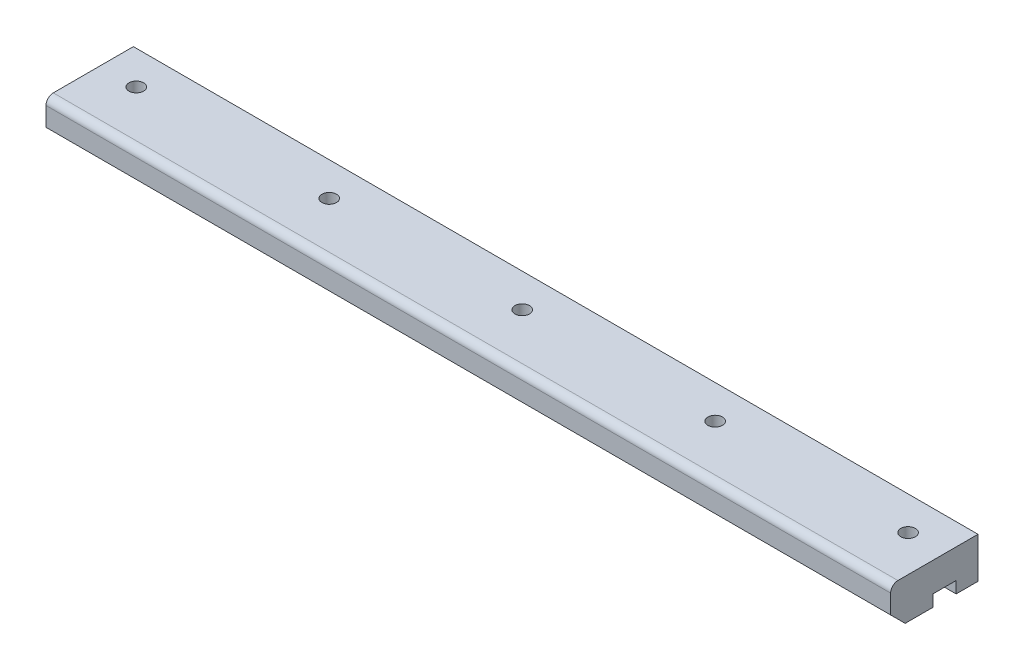
SolidWorks part; units mm, degrees
material "Plain Carbon Steel"
ref_plane "Front Plane" through (0, 0, 0) normal (0, 0, 1) x (1, 0, 0)
ref_plane "Top Plane" through (0, 0, 0) normal (0, 1, 0) x (1, 0, 0)
ref_plane "Right Plane" through (0, 0, 0) normal (1, 0, 0) x (0, 0, -1)
sketch "Rail Profile Sketch" plane through (0, 0, 0) normal (1, 0, 0) x (0, 0, -1)
  line L0 (-30, 10) -> (-30, 23)
  line L1 (-25, 28) -> (30, 28)
  line L2 (30, 28) -> (30, 0)
  line L3 (30, 0) -> (15, 0)
  line L4 (15, 0) -> (15, 8)
  line L5 (15, 8) -> (-1, 8)
  line L6 (-1, 8) -> (-1, 0)
  line L7 (-1, 0) -> (-20, 0)
  line L8 (0, 0) -> (0, 79.1227) construction
  line L9 (-20, 0) -> (-30, 10)
  arc A0 (-25, 28) -> (-30, 23) centre (-25, 23) ccw
  point P0 (-30, 0)
  point P15 (-30, 28)
  dimension "D6" = 5
  dimension "D1" = 60
  dimension "D2" = 28
  dimension "D3" = 8
  dimension "D4" = 15
  dimension "D5" = 16
extrude "Rail Body 580" add sketch "Rail Profile Sketch" along normal blind 580
sketch "Mounting Holes Sketch" plane through (0, 28, 0) normal (0, 1, 0) x (1, 0, 0)
  line L0 (0, 30) -> (0, -25) construction
  line L1 (580, 30) -> (0, 30) construction
  circle A0 centre (25, 7) radius 5
  circle A1 centre (157.5, 7) radius 5
  circle A2 centre (290, 7) radius 5
  circle A3 centre (422.5, 7) radius 5
  circle A4 centre (555, 7) radius 5
  dimension "D1" = 10
  dimension "D2" = 25
  dimension "D3" = 23
  dimension "D4" = 132.5
  dimension "D5" = 132.5
  dimension "D6" = 132.5
  dimension "D7" = 132.5
extrude "Mounting Holes 5xØ10" cut sketch "Mounting Holes Sketch" against normal blind 580
